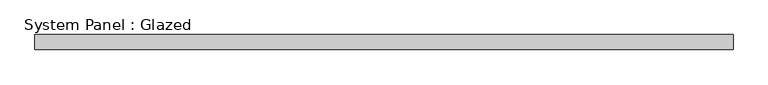
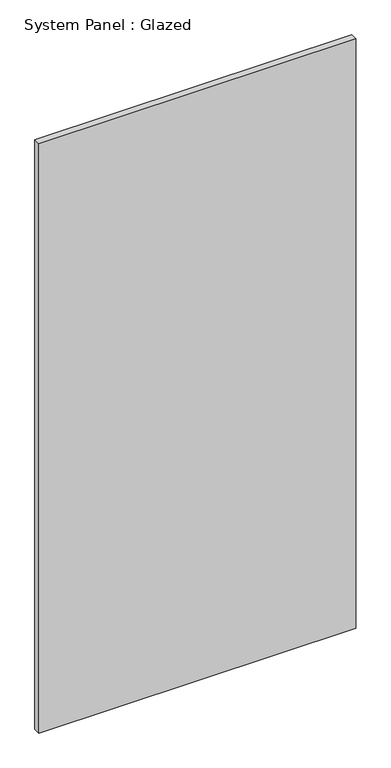
"""IFC4 building model written with IfcOpenShell, lengths in millimetres: plate geometry, System Panel : Glazed."""

from ifc_helpers import new_model, si_unit, origin, origin_with_axes, place, context, project, spatial, polyline, outline, extrude, source, transform, mapped, element, save


def system_panel_glazed_21a81833(model_context):
    return source(origin(), model_context, "Body", "SweptSolid", [
        extrude(outline(polyline([(587.6856355, 19.05), (-587.6856355, 19.05), (-587.6856355, 44.45), (587.6856355, 44.45), (587.6856355, 19.05)])), origin_with_axes(), (0.0, 0.0, 1.0), 2311.4),
    ])


if __name__ == "__main__":
    model = new_model("IFC4")
    model_context = context("Model", 3, world=origin())
    ifc_project = project(units=[si_unit("LENGTHUNIT", "METRE", prefix="MILLI")], contexts=[model_context])
    site = spatial("IfcSite", under=ifc_project)
    building = spatial("IfcBuilding", under=site)
    placement = place(None, origin())
    system_panel_glazed_shape = system_panel_glazed_21a81833(model_context)
    element("IfcPlate", 1, ObjectType="System Panel : Glazed", at=placement, inside=building, context=model_context, shape_type="MappedRepresentation", body=[
        mapped(system_panel_glazed_shape, transform((0.0, 0.0, 0.0), x_axis=(1.0, 0.0, 0.0), y_axis=(0.0, 1.0, 0.0), z_axis=(0.0, 0.0, 1.0))),
    ])
    save(model, "model.ifc")

# Revit data of these elements
# Type "System Panel : Glazed"
#   Construction Type Id = "GSP4R"
#   Analytic Construction = "1/8 in Pilkington single glazing"
#   Visual Light Transmittance = 0.9
#   Solar Heat Gain Coefficient = 0.86
#   Heat Transfer Coefficient (U) = 1.18115 BTU/(h·ft²·°F)
# Element 1 (IfcPlate, "System Panel : Glazed")
#   Materials on its faces: "Glass"
# Materials
#   "Glass": class "Glass", colour RGB 0 128 192, transparency 0.75, Description = "Soda Lime Glass", Cost = 0
